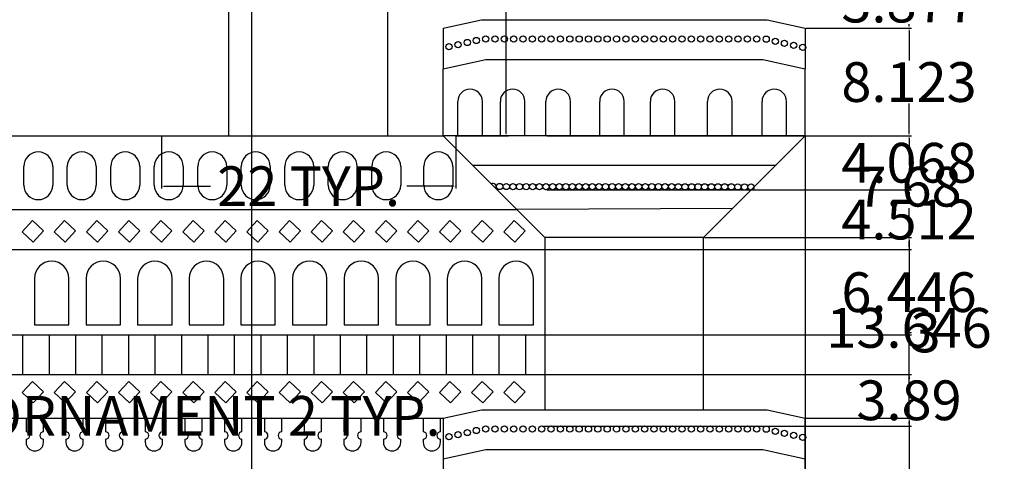
# Model space of a CAD drawing. Units: inches. Extents: x 168 to 318, y 152 to 314.
# Tile 6 of 7: x 240 to 314, y 218 to 251. Entities that reach past the tile are written whole.
import ezdxf

# ---------------------------------------------------------------- set-up
doc = ezdxf.new("R2010")
doc.units = ezdxf.units.IN
doc.header["$MEASUREMENT"] = 0
doc.layers.add('A-ANNO-DIMS', color=2, linetype='Continuous', lineweight=18)
doc.layers.add('A-ELEV', color=7, linetype='Continuous', lineweight=25)
doc.styles.get("Standard").update_dxf_attribs({"font": 'arial.ttf'})
doc.dimstyles.get("Standard").update_dxf_attribs({"dimtxt": 3, "dimasz": 0.18, "dimexe": 0.18, "dimexo": 0.0625, "dimgap": 0.09, "dimtad": 0, "dimtih": 1, "dimtoh": 1, "dimdec": 1, "dimzin": 0, "dimdsep": 46, "dimlunit": 3, "dimtxsty": 'Standard', "dimcen": 0.09, "dimadec": 0, "dimazin": 0, "dimtfac": 1, "dimtdec": 1, "dimtofl": 0, "dimtmove": 0, "dimatfit": 3, "dimfxl": 1, "dimtolj": 1, "dimtzin": 0, "dimarcsym": 0})

# ---------------------------------------------------------------- blocks, each defined once
blk = doc.blocks.new('ORN-PENDANT')
for p, q in [((0, 2.469), (0, 1.437)), ((1.31, 1.437), (1.31, 2.469)), ((0, 0.893), (0, 0.655)), ((1.31, 0.655), (1.31, 0.893))]:
    blk.add_line(p, q)
for centre, radius, start, end in [((0, 1.165), 0.272, 270, 90), ((1.31, 1.165), 0.272, 90, 270), ((0.655, 0.655), 0.655, 180, 0)]:
    blk.add_arc(centre, radius, start, end)
blk = doc.blocks.new('ARCH-BALCONY-SM')
for p, q in [((0, 0), (0, 2.603)), ((1.853, 0), (1.853, 2.603))]:
    blk.add_line(p, q)
blk.add_arc((0.926, 2.603), 0.926, 0, 180)
blk = doc.blocks.new('ARCH-ARCADE')
for p, q in [((0, 3.498), (0, 0)), ((2.6, 0), (2.6, 3.498)), ((0, 0), (2.6, 0))]:
    blk.add_line(p, q)
blk.add_arc((1.3, 3.498), 1.3, 0, 180)
blk = doc.blocks.new('OPENING-OVAL')
for p, q in [((0, 1.096), (0, 2.508)), ((2.191, 2.508), (2.191, 1.096))]:
    blk.add_line(p, q)
for centre, start, end in [((1.095, 2.508), 0, 180), ((1.095, 1.096), 180, 0)]:
    blk.add_arc(centre, 1.095, start, end)
blk = doc.blocks.new('MINARET-UPPER-STAGE')
for p, q in [((0, 24.84), (0, 22.342)), ((22.231, 24.84), (22.231, 22.343)), ((0, 18.24), (0, 22.342)), ((22.231, 18.24), (22.231, 22.342)), ((6.24, 12), (0, 18.24)), ((0, 18.24), (22.231, 18.24)), ((15.991, 12), (22.231, 18.24)), ((5.072, 0), (5.072, 12)), ((6.24, 12), (5.072, 12)), ((6.24, 12), (15.991, 12)), ((6.24, 12), (15.991, 12)), ((15.991, 12), (17.072, 12)), ((17.072, 12), (17.072, 0))]:
    blk.add_line(p, q)
for points in [[(22.231, 24.84), (19.881, 25.365), (2.344, 25.365), (0, 24.84)], [(22.231, 22.343), (19.612, 22.928), (2.613, 22.928), (0, 22.342)]]:
    blk.add_lwpolyline(points)
blk = doc.blocks.new('*D15')
at = {"layer": 'A-ANNO-DIMS', "color": 0, "lineweight": -2, "ltscale": 0.2, "transparency": 16777216}
for p, q in [((215.254, 220.875), (215.254, 221.055)), ((215.254, 221.055), (215.434, 221.055)), ((214.946, 220.875), (215.434, 220.875)), ((215.254, 218.586), (215.254, 220.695)), ((214.946, 218.406), (215.434, 218.406))]:
    blk.add_line(p, q, dxfattribs=at)
at = {"layer": 'A-ANNO-DIMS', "color": 0, "ltscale": 0.2, "transparency": 16777216}
for points in [[(215.224, 220.695), (215.284, 220.695), (215.254, 220.875)], [(215.224, 218.586), (215.284, 218.586), (215.254, 218.406)]]:
    blk.add_solid(points, dxfattribs=at)
at = {"layer": 'Defpoints', "color": 0, "ltscale": 0.2, "transparency": 16777216}
for p in [(214.883, 220.875), (215.254, 220.875), (214.883, 218.406)]:
    blk.add_point(p, dxfattribs=at)
at = {"layer": 'A-ANNO-DIMS', "color": 0, "ltscale": 0.2, "transparency": 16777216, "insert": (244.753, 221.055), "char_height": 3, "attachment_point": 5}
blk.add_mtext('\\A1;PENDANT ORNAMENT 2 TYP.', dxfattribs=at)
blk = doc.blocks.new('*D23')
at = {"layer": 'A-ANNO-DIMS', "color": 0, "lineweight": -2, "ltscale": 0.2, "transparency": 16777216}
for p, q in [((261.882, 214.562), (263.075, 214.562)), ((262.895, 214.382), (262.895, 212.619)), ((262.895, 207.574), (262.895, 209.337)), ((261.882, 207.394), (263.075, 207.394))]:
    blk.add_line(p, q, dxfattribs=at)
at = {"layer": 'A-ANNO-DIMS', "color": 0, "ltscale": 0.2, "transparency": 16777216}
for points in [[(262.865, 214.382), (262.925, 214.382), (262.895, 214.562)], [(262.865, 207.574), (262.925, 207.574), (262.895, 207.394)]]:
    blk.add_solid(points, dxfattribs=at)
at = {"layer": 'Defpoints', "color": 0, "ltscale": 0.2, "transparency": 16777216}
for p in [(261.82, 214.562), (262.895, 214.562), (261.82, 207.394)]:
    blk.add_point(p, dxfattribs=at)
at = {"layer": 'A-ANNO-DIMS', "color": 0, "ltscale": 0.2, "transparency": 16777216, "insert": (262.895, 210.978), "char_height": 3, "attachment_point": 5}
blk.add_mtext('\\A1;CUSPED ARCH PANEL 7 TYP.', dxfattribs=at)
blk = doc.blocks.new('*D25')
at = {"layer": 'A-ANNO-DIMS', "color": 0, "lineweight": -2, "ltscale": 0.2, "transparency": 16777216}
for p, q in [((273.097, 267.566), (277.02, 267.566)), ((276.84, 267.386), (276.84, 256.525)), ((276.84, 242.381), (276.84, 253.243)), ((273.097, 242.201), (277.02, 242.201))]:
    blk.add_line(p, q, dxfattribs=at)
at = {"layer": 'A-ANNO-DIMS', "color": 0, "ltscale": 0.2, "transparency": 16777216}
for points in [[(276.81, 267.386), (276.87, 267.386), (276.84, 267.566)], [(276.81, 242.381), (276.87, 242.381), (276.84, 242.201)]]:
    blk.add_solid(points, dxfattribs=at)
at = {"layer": 'Defpoints', "color": 0, "ltscale": 0.2, "transparency": 16777216}
for p in [(273.035, 267.566), (276.84, 267.566), (273.035, 242.201)]:
    blk.add_point(p, dxfattribs=at)
at = {"layer": 'A-ANNO-DIMS', "color": 0, "ltscale": 0.2, "transparency": 16777216, "insert": (276.84, 254.884), "char_height": 3, "attachment_point": 5}
blk.add_mtext('\\A1;MINARET UPPER STAGE 25 TYP.', dxfattribs=at)
blk = doc.blocks.new('*D26')
at = {"layer": 'A-ANNO-DIMS', "color": 0, "lineweight": -2, "ltscale": 0.2, "transparency": 16777216}
for p, q in [((250.804, 242.139), (250.804, 238.217)), ((273.035, 242.139), (273.035, 238.217)), ((250.984, 238.397), (254.502, 238.397)), ((272.855, 238.397), (269.337, 238.397))]:
    blk.add_line(p, q, dxfattribs=at)
at = {"layer": 'A-ANNO-DIMS', "color": 0, "ltscale": 0.2, "transparency": 16777216}
for points in [[(250.984, 238.427), (250.984, 238.367), (250.804, 238.397)], [(272.855, 238.427), (272.855, 238.367), (273.035, 238.397)]]:
    blk.add_solid(points, dxfattribs=at)
at = {"layer": 'Defpoints', "color": 0, "ltscale": 0.2, "transparency": 16777216}
for p in [(250.804, 242.201), (273.035, 242.201), (273.035, 238.397)]:
    blk.add_point(p, dxfattribs=at)
at = {"layer": 'A-ANNO-DIMS', "color": 0, "ltscale": 0.2, "transparency": 16777216, "insert": (261.92, 238.397), "char_height": 3, "attachment_point": 5}
blk.add_mtext('\\A1;22 TYP.', dxfattribs=at)
blk = doc.blocks.new('*D29')
at = {"layer": 'A-ANNO-DIMS', "color": 0, "lineweight": -2, "ltscale": 0.2, "transparency": 16777216}
for p, q in [((184.724, 242.139), (184.724, 154.215)), ((299.445, 242.139), (299.445, 154.215)), ((184.904, 154.395), (235.924, 154.395)), ((299.265, 154.395), (248.245, 154.395))]:
    blk.add_line(p, q, dxfattribs=at)
at = {"layer": 'A-ANNO-DIMS', "color": 0, "ltscale": 0.2, "transparency": 16777216}
for points in [[(184.904, 154.425), (184.904, 154.365), (184.724, 154.395)], [(299.265, 154.425), (299.265, 154.365), (299.445, 154.395)]]:
    blk.add_solid(points, dxfattribs=at)
at = {"layer": 'Defpoints', "color": 0, "ltscale": 0.2, "transparency": 16777216}
for p in [(184.724, 242.201), (299.445, 242.201), (299.445, 154.395)]:
    blk.add_point(p, dxfattribs=at)
at = {"layer": 'A-ANNO-DIMS', "color": 0, "ltscale": 0.2, "transparency": 16777216, "insert": (242.084, 154.395), "char_height": 3, "attachment_point": 5}
blk.add_mtext('\\A1;114.72', dxfattribs=at)
blk = doc.blocks.new('*D36')
at = {"layer": 'A-ANNO-DIMS', "color": 0, "lineweight": -2, "ltscale": 0.2, "transparency": 16777216}
for p, q in [((299.507, 220.875), (307.468, 220.875)), ((307.288, 220.695), (307.288, 214.997)), ((307.288, 206.055), (307.288, 211.754)), ((299.507, 205.875), (307.468, 205.875))]:
    blk.add_line(p, q, dxfattribs=at)
at = {"layer": 'A-ANNO-DIMS', "color": 0, "ltscale": 0.2, "transparency": 16777216}
for points in [[(307.258, 220.695), (307.318, 220.695), (307.288, 220.875)], [(307.258, 206.055), (307.318, 206.055), (307.288, 205.875)]]:
    blk.add_solid(points, dxfattribs=at)
at = {"layer": 'Defpoints', "color": 0, "ltscale": 0.2, "transparency": 16777216}
for p in [(299.445, 220.875), (307.288, 220.875), (299.445, 205.875)]:
    blk.add_point(p, dxfattribs=at)
at = {"layer": 'A-ANNO-DIMS', "color": 0, "ltscale": 0.2, "transparency": 16777216, "insert": (307.288, 213.375), "char_height": 3, "attachment_point": 5}
blk.add_mtext('\\A1;15', dxfattribs=at)
blk = doc.blocks.new('*D37')
at = {"layer": 'A-ANNO-DIMS', "color": 0, "lineweight": -2, "ltscale": 0.2, "transparency": 16777216}
for p, q in [((291.827, 234.521), (307.468, 234.521)), ((307.288, 234.341), (307.288, 229.321)), ((307.288, 221.055), (307.288, 226.076)), ((299.507, 220.875), (307.468, 220.875))]:
    blk.add_line(p, q, dxfattribs=at)
at = {"layer": 'A-ANNO-DIMS', "color": 0, "ltscale": 0.2, "transparency": 16777216}
for points in [[(307.258, 234.341), (307.318, 234.341), (307.288, 234.521)], [(307.258, 221.055), (307.318, 221.055), (307.288, 220.875)]]:
    blk.add_solid(points, dxfattribs=at)
at = {"layer": 'Defpoints', "color": 0, "ltscale": 0.2, "transparency": 16777216}
for p in [(291.765, 234.521), (307.288, 234.521), (299.445, 220.875)]:
    blk.add_point(p, dxfattribs=at)
at = {"layer": 'A-ANNO-DIMS', "color": 0, "ltscale": 0.2, "transparency": 16777216, "insert": (307.288, 227.698), "char_height": 3, "attachment_point": 5}
blk.add_mtext('\\A1;13.646', dxfattribs=at)
blk = doc.blocks.new('*D38')
at = {"layer": 'A-ANNO-DIMS', "color": 0, "lineweight": -2, "ltscale": 0.2, "transparency": 16777216}
for p, q in [((299.507, 242.201), (307.468, 242.201)), ((307.288, 242.021), (307.288, 239.983)), ((307.288, 234.701), (307.288, 236.74)), ((291.827, 234.521), (307.468, 234.521))]:
    blk.add_line(p, q, dxfattribs=at)
at = {"layer": 'A-ANNO-DIMS', "color": 0, "ltscale": 0.2, "transparency": 16777216}
for points in [[(307.258, 242.021), (307.318, 242.021), (307.288, 242.201)], [(307.258, 234.701), (307.318, 234.701), (307.288, 234.521)]]:
    blk.add_solid(points, dxfattribs=at)
at = {"layer": 'Defpoints', "color": 0, "ltscale": 0.2, "transparency": 16777216}
for p in [(299.445, 242.201), (307.288, 242.201), (291.765, 234.521)]:
    blk.add_point(p, dxfattribs=at)
at = {"layer": 'A-ANNO-DIMS', "color": 0, "ltscale": 0.2, "transparency": 16777216, "insert": (307.288, 238.361), "char_height": 3, "attachment_point": 5}
blk.add_mtext('\\A1;7.68', dxfattribs=at)
blk = doc.blocks.new('*D39')
at = {"layer": 'A-ANNO-DIMS', "color": 0, "lineweight": -2, "ltscale": 0.2, "transparency": 16777216}
for p, q in [((299.507, 250.324), (307.468, 250.324)), ((307.288, 250.144), (307.288, 247.886)), ((307.288, 242.381), (307.288, 244.64)), ((299.507, 242.201), (307.468, 242.201))]:
    blk.add_line(p, q, dxfattribs=at)
at = {"layer": 'A-ANNO-DIMS', "color": 0, "ltscale": 0.2, "transparency": 16777216}
for points in [[(307.258, 250.144), (307.318, 250.144), (307.288, 250.324)], [(307.258, 242.381), (307.318, 242.381), (307.288, 242.201)]]:
    blk.add_solid(points, dxfattribs=at)
at = {"layer": 'Defpoints', "color": 0, "ltscale": 0.2, "transparency": 16777216}
for p in [(299.445, 250.324), (307.288, 250.324), (299.445, 242.201)]:
    blk.add_point(p, dxfattribs=at)
at = {"layer": 'A-ANNO-DIMS', "color": 0, "ltscale": 0.2, "transparency": 16777216, "insert": (307.288, 246.263), "char_height": 3, "attachment_point": 5}
blk.add_mtext('\\A1;8.123', dxfattribs=at)
blk = doc.blocks.new('*D40')
at = {"layer": 'A-ANNO-DIMS', "color": 0, "lineweight": -2, "ltscale": 0.2, "transparency": 16777216}
for p, q in [((267.939, 254.201), (307.468, 254.201)), ((307.288, 254.021), (307.288, 253.886)), ((299.507, 250.324), (307.468, 250.324)), ((307.288, 250.504), (307.288, 250.64))]:
    blk.add_line(p, q, dxfattribs=at)
at = {"layer": 'A-ANNO-DIMS', "color": 0, "ltscale": 0.2, "transparency": 16777216}
for points in [[(307.258, 254.021), (307.318, 254.021), (307.288, 254.201)], [(307.258, 250.504), (307.318, 250.504), (307.288, 250.324)]]:
    blk.add_solid(points, dxfattribs=at)
at = {"layer": 'Defpoints', "color": 0, "ltscale": 0.2, "transparency": 16777216}
for p in [(267.877, 254.201), (307.288, 254.201), (299.445, 250.324)]:
    blk.add_point(p, dxfattribs=at)
at = {"layer": 'A-ANNO-DIMS', "color": 0, "ltscale": 0.2, "transparency": 16777216, "insert": (307.288, 252.263), "char_height": 3, "attachment_point": 5}
blk.add_mtext('\\A1;3.877', dxfattribs=at)
blk = doc.blocks.new('*D57')
at = {"layer": 'A-ANNO-DIMS', "color": 0, "lineweight": -2, "ltscale": 0.2, "transparency": 16777216}
for p, q in [((226.54, 195.647), (226.54, 312.411)), ((226.72, 312.231), (236.931, 312.231)), ((257.449, 312.231), (247.238, 312.231)), ((257.629, 195.647), (257.629, 312.411))]:
    blk.add_line(p, q, dxfattribs=at)
at = {"layer": 'A-ANNO-DIMS', "color": 0, "ltscale": 0.2, "transparency": 16777216}
for points in [[(226.72, 312.261), (226.72, 312.201), (226.54, 312.231)], [(257.449, 312.261), (257.449, 312.201), (257.629, 312.231)]]:
    blk.add_solid(points, dxfattribs=at)
at = {"layer": 'Defpoints', "color": 0, "ltscale": 0.2, "transparency": 16777216}
for p in [(257.629, 312.231), (226.54, 195.584), (257.629, 195.584)]:
    blk.add_point(p, dxfattribs=at)
at = {"layer": 'A-ANNO-DIMS', "color": 0, "ltscale": 0.2, "transparency": 16777216, "insert": (242.084, 312.231), "char_height": 3, "attachment_point": 5}
blk.add_mtext('\\A1;31.09', dxfattribs=at)
blk = doc.blocks.new('*D76')
at = {"layer": 'A-ANNO-DIMS', "color": 0, "lineweight": -2, "ltscale": 0.2, "transparency": 16777216}
for p, q in [((279.689, 220.29), (307.468, 220.29)), ((307.288, 220.11), (307.288, 215.463)), ((307.288, 207.574), (307.288, 212.22)), ((272.147, 207.394), (307.468, 207.394))]:
    blk.add_line(p, q, dxfattribs=at)
at = {"layer": 'A-ANNO-DIMS', "color": 0, "ltscale": 0.2, "transparency": 16777216}
for points in [[(307.258, 220.11), (307.318, 220.11), (307.288, 220.29)], [(307.258, 207.574), (307.318, 207.574), (307.288, 207.394)]]:
    blk.add_solid(points, dxfattribs=at)
at = {"layer": 'Defpoints', "color": 0, "ltscale": 0.2, "transparency": 16777216}
for p in [(279.627, 220.29), (307.288, 220.29), (272.084, 207.394)]:
    blk.add_point(p, dxfattribs=at)
at = {"layer": 'A-ANNO-DIMS', "color": 0, "ltscale": 0.2, "transparency": 16777216, "insert": (307.288, 213.842), "char_height": 3, "attachment_point": 5}
blk.add_mtext('\\A1;12.896', dxfattribs=at)
blk = doc.blocks.new('*D77')
at = {"layer": 'A-ANNO-DIMS', "color": 0, "lineweight": -2, "ltscale": 0.2, "transparency": 16777216}
for p, q in [((279.827, 224.175), (307.468, 224.175)), ((307.288, 223.995), (307.288, 223.855)), ((279.689, 220.29), (307.468, 220.29)), ((307.288, 220.47), (307.288, 220.61))]:
    blk.add_line(p, q, dxfattribs=at)
at = {"layer": 'A-ANNO-DIMS', "color": 0, "ltscale": 0.2, "transparency": 16777216}
for points in [[(307.258, 223.995), (307.318, 223.995), (307.288, 224.175)], [(307.258, 220.47), (307.318, 220.47), (307.288, 220.29)]]:
    blk.add_solid(points, dxfattribs=at)
at = {"layer": 'Defpoints', "color": 0, "ltscale": 0.2, "transparency": 16777216}
for p in [(279.765, 224.175), (307.288, 224.175), (279.627, 220.29)]:
    blk.add_point(p, dxfattribs=at)
at = {"layer": 'A-ANNO-DIMS', "color": 0, "ltscale": 0.2, "transparency": 16777216, "insert": (307.288, 222.232), "char_height": 3, "attachment_point": 5}
blk.add_mtext('\\A1;3.89', dxfattribs=at)
blk = doc.blocks.new('*D78')
at = {"layer": 'A-ANNO-DIMS', "color": 0, "lineweight": -2, "ltscale": 0.2, "transparency": 16777216}
for p, q in [((279.827, 227.175), (307.468, 227.175)), ((307.288, 227.175), (307.288, 227.355)), ((307.288, 227.355), (307.468, 227.355)), ((307.288, 224.355), (307.288, 226.995)), ((279.827, 224.175), (307.468, 224.175))]:
    blk.add_line(p, q, dxfattribs=at)
at = {"layer": 'A-ANNO-DIMS', "color": 0, "ltscale": 0.2, "transparency": 16777216}
for points in [[(307.258, 226.995), (307.318, 226.995), (307.288, 227.175)], [(307.258, 224.355), (307.318, 224.355), (307.288, 224.175)]]:
    blk.add_solid(points, dxfattribs=at)
at = {"layer": 'Defpoints', "color": 0, "ltscale": 0.2, "transparency": 16777216}
for p in [(279.765, 227.175), (307.288, 227.175), (279.765, 224.175)]:
    blk.add_point(p, dxfattribs=at)
at = {"layer": 'A-ANNO-DIMS', "color": 0, "ltscale": 0.2, "transparency": 16777216, "insert": (308.541, 227.355), "char_height": 3, "attachment_point": 5}
blk.add_mtext('\\A1;3', dxfattribs=at)
blk = doc.blocks.new('*D79')
at = {"layer": 'A-ANNO-DIMS', "color": 0, "lineweight": -2, "ltscale": 0.2, "transparency": 16777216}
for p, q in [((279.827, 233.621), (307.468, 233.621)), ((307.288, 233.441), (307.288, 232.02)), ((307.288, 227.355), (307.288, 228.776)), ((279.827, 227.175), (307.468, 227.175))]:
    blk.add_line(p, q, dxfattribs=at)
at = {"layer": 'A-ANNO-DIMS', "color": 0, "ltscale": 0.2, "transparency": 16777216}
for points in [[(307.258, 233.441), (307.318, 233.441), (307.288, 233.621)], [(307.258, 227.355), (307.318, 227.355), (307.288, 227.175)]]:
    blk.add_solid(points, dxfattribs=at)
at = {"layer": 'Defpoints', "color": 0, "ltscale": 0.2, "transparency": 16777216}
for p in [(279.765, 233.621), (307.288, 233.621), (279.765, 227.175)]:
    blk.add_point(p, dxfattribs=at)
at = {"layer": 'A-ANNO-DIMS', "color": 0, "ltscale": 0.2, "transparency": 16777216, "insert": (307.288, 230.398), "char_height": 3, "attachment_point": 5}
blk.add_mtext('\\A1;6.446', dxfattribs=at)
blk = doc.blocks.new('*D80')
at = {"layer": 'A-ANNO-DIMS', "color": 0, "lineweight": -2, "ltscale": 0.2, "transparency": 16777216}
for p, q in [((279.917, 238.133), (307.468, 238.133)), ((307.288, 237.953), (307.288, 237.499)), ((307.288, 233.801), (307.288, 234.255)), ((279.827, 233.621), (307.468, 233.621))]:
    blk.add_line(p, q, dxfattribs=at)
at = {"layer": 'A-ANNO-DIMS', "color": 0, "ltscale": 0.2, "transparency": 16777216}
for points in [[(307.258, 237.953), (307.318, 237.953), (307.288, 238.133)], [(307.258, 233.801), (307.318, 233.801), (307.288, 233.621)]]:
    blk.add_solid(points, dxfattribs=at)
at = {"layer": 'Defpoints', "color": 0, "ltscale": 0.2, "transparency": 16777216}
for p in [(279.854, 238.133), (307.288, 238.133), (279.765, 233.621)]:
    blk.add_point(p, dxfattribs=at)
at = {"layer": 'A-ANNO-DIMS', "color": 0, "ltscale": 0.2, "transparency": 16777216, "insert": (307.288, 235.877), "char_height": 3, "attachment_point": 5}
blk.add_mtext('\\A1;4.512', dxfattribs=at)
blk = doc.blocks.new('*D81')
at = {"layer": 'A-ANNO-DIMS', "color": 0, "lineweight": -2, "ltscale": 0.2, "transparency": 16777216}
for p, q in [((279.916, 242.201), (307.468, 242.201)), ((307.288, 242.021), (307.288, 241.789)), ((279.917, 238.133), (307.468, 238.133)), ((307.288, 238.313), (307.288, 238.545))]:
    blk.add_line(p, q, dxfattribs=at)
at = {"layer": 'A-ANNO-DIMS', "color": 0, "ltscale": 0.2, "transparency": 16777216}
for points in [[(307.258, 242.021), (307.318, 242.021), (307.288, 242.201)], [(307.258, 238.313), (307.318, 238.313), (307.288, 238.133)]]:
    blk.add_solid(points, dxfattribs=at)
at = {"layer": 'Defpoints', "color": 0, "ltscale": 0.2, "transparency": 16777216}
for p in [(279.854, 242.201), (307.288, 242.201), (279.854, 238.133)]:
    blk.add_point(p, dxfattribs=at)
at = {"layer": 'A-ANNO-DIMS', "color": 0, "ltscale": 0.2, "transparency": 16777216, "insert": (307.288, 240.167), "char_height": 3, "attachment_point": 5}
blk.add_mtext('\\A1;4.068', dxfattribs=at)

msp = doc.modelspace()

# ---------------------------------------------------------------- linework, layer by layer
at = {"layer": 'A-ELEV'}
for p, q in [((272.0845, 250.3243), (272.0845, 247.2504)), ((299.4446, 250.3243), (299.4446, 247.25)), ((272.0845, 242.2013), (272.0845, 247.25)), ((299.4446, 242.2013), (299.4446, 247.25)), ((212.0845, 242.2013), (272.0845, 242.2013)), ((299.4446, 242.2013), (272.0845, 242.2013)), ((279.7645, 234.5213), (272.0845, 242.2013)), ((291.7645, 234.5213), (299.4446, 242.2013)), ((297.2168, 239.9735), (274.3285, 239.9573)), ((206.511, 236.6279), (277.6579, 236.6279)), ((293.9532, 236.7099), (277.6579, 236.6279)), ((279.7645, 234.5213), (279.7645, 221.5213)), ((291.7645, 234.5213), (279.7645, 234.5213)), ((291.7645, 221.5213), (291.7645, 234.5213)), ((204.4044, 233.6213), (279.7645, 233.6213)), ((204.4044, 227.1751), (279.7645, 227.1751)), ((240.3013, 227.1751), (240.3013, 224.1751)), ((242.3013, 227.1751), (242.3013, 224.1751)), ((244.3013, 227.1751), (244.3013, 224.1751)), ((246.3013, 227.1751), (246.3013, 224.1751)), ((248.3013, 227.1751), (248.3013, 224.1751)), ((250.3013, 227.1751), (250.3013, 224.1751)), ((252.3013, 227.1751), (252.3013, 224.1751)), ((254.3013, 227.1751), (254.3013, 224.1751)), ((256.3013, 227.1751), (256.3013, 224.1751)), ((258.3013, 227.1751), (258.3013, 224.1751)), ((260.3013, 227.1751), (260.3013, 224.1751)), ((262.3013, 227.1751), (262.3013, 224.1751)), ((264.3013, 227.1751), (264.3013, 224.1751)), ((266.3013, 227.1751), (266.3013, 224.1751)), ((268.3013, 227.1751), (268.3013, 224.1751)), ((270.3013, 227.1751), (270.3013, 224.1751)), ((272.3013, 227.1751), (272.3013, 224.1751)), ((274.3013, 227.1751), (274.3013, 224.1751)), ((276.3013, 227.1751), (276.3013, 224.1751)), ((278.3013, 227.1751), (278.3013, 224.1751)), ((204.4044, 224.1751), (279.7645, 224.1751)), ((212.0845, 220.8755), (272.0845, 220.8755)), ((272.0845, 220.8755), (272.0845, 205.8755)), ((299.4446, 205.8755), (299.4446, 220.8755))]:
    msp.add_line(p, q, dxfattribs=at)
for points in [[(272.0845, 250.3243), (274.976, 250.9701), (296.5602, 250.9701), (299.4446, 250.3243)], [(272.0845, 247.2504), (275.3069, 247.9701), (296.2285, 247.9701), (299.4446, 247.25)], [(272.0845, 220.8755), (274.976, 221.5213), (296.5602, 221.5213), (299.4446, 220.8755)], [(272.0845, 217.8016), (275.3069, 218.5213), (296.2285, 218.5213), (299.4446, 217.8012)]]:
    msp.add_lwpolyline(points, dxfattribs=at)
for points in [[(241.8881, 235.0162), (241.0529, 235.7986), (240.2706, 234.9634), (241.1057, 234.1811)], [(244.3143, 235.0162), (243.4792, 235.7986), (242.6968, 234.9634), (243.532, 234.1811)], [(246.7406, 235.0162), (245.9054, 235.7986), (245.1231, 234.9634), (245.9582, 234.1811)], [(249.1668, 235.0162), (248.3317, 235.7986), (247.5493, 234.9634), (248.3845, 234.1811)], [(251.5931, 235.0162), (250.7579, 235.7986), (249.9756, 234.9634), (250.8108, 234.1811)], [(254.0194, 235.0162), (253.1842, 235.7986), (252.4019, 234.9634), (253.237, 234.1811)], [(256.4456, 235.0162), (255.6105, 235.7986), (254.8281, 234.9634), (255.6633, 234.1811)], [(258.8719, 235.0162), (258.0367, 235.7986), (257.2544, 234.9634), (258.0896, 234.1811)], [(261.2982, 235.0162), (260.463, 235.7986), (259.6806, 234.9634), (260.5158, 234.1811)], [(263.7244, 235.0162), (262.8892, 235.7986), (262.1069, 234.9634), (262.9421, 234.1811)], [(266.1507, 235.0162), (265.3155, 235.7986), (264.5332, 234.9634), (265.3683, 234.1811)], [(268.5769, 235.0162), (267.7418, 235.7986), (266.9594, 234.9634), (267.7946, 234.1811)], [(271.0032, 235.0162), (270.168, 235.7986), (269.3857, 234.9634), (270.2209, 234.1811)], [(273.4295, 235.0162), (272.5943, 235.7986), (271.812, 234.9634), (272.6471, 234.1811)], [(275.8557, 235.0162), (275.0206, 235.7986), (274.2382, 234.9634), (275.0734, 234.1811)], [(278.282, 235.0162), (277.4468, 235.7986), (276.6645, 234.9634), (277.4996, 234.1811)], [(241.8881, 222.8812), (241.0529, 223.6635), (240.2706, 222.8284), (241.1057, 222.046)], [(244.3143, 222.8812), (243.4792, 223.6635), (242.6968, 222.8284), (243.532, 222.046)], [(246.7406, 222.8812), (245.9054, 223.6635), (245.1231, 222.8284), (245.9582, 222.046)], [(249.1668, 222.8812), (248.3317, 223.6635), (247.5493, 222.8284), (248.3845, 222.046)], [(251.5931, 222.8812), (250.7579, 223.6635), (249.9756, 222.8284), (250.8108, 222.046)], [(254.0194, 222.8812), (253.1842, 223.6635), (252.4019, 222.8284), (253.237, 222.046)], [(256.4456, 222.8812), (255.6105, 223.6635), (254.8281, 222.8284), (255.6633, 222.046)], [(258.8719, 222.8812), (258.0367, 223.6635), (257.2544, 222.8284), (258.0896, 222.046)], [(261.2982, 222.8812), (260.463, 223.6635), (259.6806, 222.8284), (260.5158, 222.046)], [(263.7244, 222.8812), (262.8892, 223.6635), (262.1069, 222.8284), (262.9421, 222.046)], [(266.1507, 222.8812), (265.3155, 223.6635), (264.5332, 222.8284), (265.3683, 222.046)], [(268.5769, 222.8812), (267.7418, 223.6635), (266.9594, 222.8284), (267.7946, 222.046)], [(271.0032, 222.8812), (270.168, 223.6635), (269.3857, 222.8284), (270.2209, 222.046)], [(273.4295, 222.8812), (272.5943, 223.6635), (271.812, 222.8284), (272.6471, 222.046)], [(275.8557, 222.8812), (275.0206, 223.6635), (274.2382, 222.8284), (275.0734, 222.046)], [(278.282, 222.8812), (277.4468, 223.6635), (276.6645, 222.8284), (277.4996, 222.046)]]:
    msp.add_lwpolyline(points, close=True, dxfattribs=at)
for centre in [(273.2141, 249.0923), (273.9034, 249.2463), (274.5928, 249.4003), (275.2971, 249.5215), (276.0034, 249.5215), (276.7097, 249.5215), (277.4161, 249.5215), (278.1224, 249.5215), (278.8287, 249.5215), (279.535, 249.5215), (280.2414, 249.5215), (280.9477, 249.5215), (281.654, 249.5215), (282.3604, 249.5215), (283.0667, 249.5215), (283.773, 249.5215), (284.4793, 249.5215), (285.1857, 249.5215), (285.892, 249.5215), (286.5983, 249.5215), (287.3047, 249.5215), (288.011, 249.5215), (288.7173, 249.5215), (289.4236, 249.5215), (290.13, 249.5215), (290.8363, 249.5215), (291.5426, 249.5215), (292.249, 249.5215), (292.9553, 249.5215), (293.6616, 249.5215), (294.3679, 249.5215), (295.0743, 249.5215), (295.7806, 249.5215), (296.4959, 249.5001), (297.1852, 249.3457), (297.8745, 249.1914), (298.5637, 249.0371), (272.5247, 248.9384), (299.253, 248.8828), (276.354, 238.3735), (276.854, 238.3728), (277.354, 238.372), (277.854, 238.3713), (278.354, 238.3706), (278.854, 238.3699), (279.354, 238.3692), (279.854, 238.3685), (280.354, 238.3677), (280.854, 238.367), (281.354, 238.3663), (281.854, 238.3656), (282.354, 238.3649), (282.854, 238.3642), (283.354, 238.3634), (283.854, 238.3627), (284.354, 238.362), (284.854, 238.3613), (285.354, 238.3606), (285.854, 238.3599), (286.354, 238.3591), (286.854, 238.3584), (287.354, 238.3577), (287.854, 238.357), (288.354, 238.3563), (288.854, 238.3556), (289.354, 238.3548), (289.854, 238.3541), (290.354, 238.3534), (290.854, 238.3527), (291.354, 238.352), (291.854, 238.3513), (292.354, 238.3505), (292.854, 238.3498), (293.354, 238.3491), (293.854, 238.3484), (294.354, 238.3477), (294.854, 238.347), (295.354, 238.3462), (275.2971, 220.0727), (276.0034, 220.0727), (276.7097, 220.0727), (277.4161, 220.0727), (278.1224, 220.0727), (278.8287, 220.0727), (279.535, 220.0727), (280.2414, 220.0727), (280.9477, 220.0727), (281.654, 220.0727), (282.3604, 220.0727), (283.0667, 220.0727), (283.773, 220.0727), (284.4793, 220.0727), (285.1857, 220.0727), (285.892, 220.0727), (286.5983, 220.0727), (287.3047, 220.0727), (288.011, 220.0727), (288.7173, 220.0727), (289.4236, 220.0727), (290.13, 220.0727), (290.8363, 220.0727), (291.5426, 220.0727), (292.249, 220.0727), (292.9553, 220.0727), (293.6616, 220.0727), (294.3679, 220.0727), (295.0743, 220.0727), (295.7806, 220.0727), (296.4959, 220.0513), (272.5247, 219.4896), (273.2141, 219.6435), (273.9034, 219.7975), (274.5928, 219.9515), (297.1852, 219.8969), (297.8745, 219.7426), (298.5637, 219.5883), (299.253, 219.434)]:
    msp.add_circle(centre, 0.2354, dxfattribs=at)
msp.add_arc((275.854, 238.3742), 0.2354, 324.95912, 125.04088, dxfattribs=at)

# ---------------------------------------------------------------- block references
for name, p in [('MINARET-UPPER-STAGE', (250.8041, 242.2012)), ('ARCH-BALCONY-SM', (273.1935, 242.2009)), ('ARCH-BALCONY-SM', (276.4067, 242.2009)), ('ARCH-BALCONY-SM', (279.8536, 242.2009)), ('ARCH-BALCONY-SM', (283.9118, 242.2009)), ('ARCH-BALCONY-SM', (287.7406, 242.2009)), ('ARCH-BALCONY-SM', (292.0638, 242.2009)), ('ARCH-BALCONY-SM', (296.1823, 242.2009)), ('OPENING-OVAL', (240.3947, 237.381)), ('OPENING-OVAL', (243.6811, 237.381)), ('OPENING-OVAL', (246.9676, 237.381)), ('OPENING-OVAL', (250.254, 237.381)), ('OPENING-OVAL', (253.5404, 237.381)), ('OPENING-OVAL', (256.8268, 237.381)), ('OPENING-OVAL', (260.1132, 237.381)), ('OPENING-OVAL', (263.3996, 237.381)), ('OPENING-OVAL', (266.686, 237.381)), ('OPENING-OVAL', (270.6196, 237.3808)), ('ARCH-ARCADE', (241.199, 227.938)), ('ARCH-ARCADE', (245.099, 227.938)), ('ARCH-ARCADE', (248.999, 227.938)), ('ARCH-ARCADE', (252.899, 227.938)), ('ARCH-ARCADE', (256.799, 227.938)), ('ARCH-ARCADE', (260.699, 227.938)), ('ARCH-ARCADE', (264.599, 227.938)), ('ARCH-ARCADE', (268.499, 227.938)), ('ARCH-ARCADE', (272.399, 227.938)), ('ARCH-ARCADE', (276.299, 227.938)), ('ORN-PENDANT', (240.573, 218.406)), ('ORN-PENDANT', (243.573, 218.406)), ('ORN-PENDANT', (246.573, 218.406)), ('ORN-PENDANT', (249.573, 218.406)), ('ORN-PENDANT', (252.573, 218.406)), ('ORN-PENDANT', (255.573, 218.406)), ('ORN-PENDANT', (258.573, 218.406)), ('ORN-PENDANT', (261.573, 218.406)), ('ORN-PENDANT', (264.573, 218.406)), ('ORN-PENDANT', (267.573, 218.406)), ('ORN-PENDANT', (270.573, 218.406))]:
    msp.add_blockref(name, p, dxfattribs=at)

# ---------------------------------------------------------------- dimensions: what is measured, and where the dimension line sits
at = {"layer": 'A-ANNO-DIMS', "ltscale": 0.2}
for base, p1, p2, picture, middle in [((257.6286, 312.2308), (226.5403, 195.5844), (257.6286, 195.5844), '*D57', (242.0845, 312.2308)), ((299.4446, 154.3954), (184.7244, 242.2013), (299.4446, 242.2013), '*D29', (242.0845, 154.3954))]:
    dim = msp.add_linear_dim(base=base, p1=p1, p2=p2, dimstyle='Standard', override={"dimdec": 2, "dimlfac": 1, "dimrnd": 0, "dimzin": 0, "dimdsep": 46, "dimlunit": 2}, dxfattribs=at)
    dim.commit()
    dim.dimension.update_dxf_attribs({"geometry": picture, "text_midpoint": middle})
for base, p1, p2, text, picture, middle in [((276.8396, 267.5663), (273.0348, 242.2013), (273.0348, 267.5663), 'MINARET UPPER STAGE <> TYP.', '*D25', (276.8396, 254.8838)), ((215.2539, 220.8755), (214.8834, 218.4056), (214.8834, 220.8755), 'PENDANT ORNAMENT <> TYP.', '*D15', (244.7534, 221.0555)), ((262.8949, 214.5622), (261.8196, 207.3935), (261.8196, 214.5622), 'CUSPED ARCH PANEL <> TYP.', '*D23', (262.8949, 210.9778))]:
    dim = msp.add_linear_dim(base=base, p1=p1, p2=p2, angle=90, text=text, dimstyle='Standard', override={"dimdec": 0, "dimrnd": 0, "dimzin": 0, "dimlunit": 2}, dxfattribs=at)
    dim.commit()
    dim.dimension.update_dxf_attribs({"geometry": picture, "text_midpoint": middle})
for base, p1, p2, override, picture, middle in [((307.2884, 254.2013), (299.4446, 250.3243), (267.8765, 254.2013), {"dimdec": 3, "dimlfac": 1, "dimrnd": 0, "dimzin": 0, "dimdsep": 46, "dimlunit": 2}, '*D40', (307.2884, 252.2628)), ((307.2884, 250.3243), (299.4446, 242.2013), (299.4446, 250.3243), {"dimdec": 3, "dimlfac": 1, "dimrnd": 0, "dimzin": 0, "dimdsep": 46, "dimlunit": 2}, '*D39', (307.2884, 246.2628)), ((307.2884, 242.2013), (279.854, 238.133), (279.8535, 242.2013), {"dimdec": 3, "dimlfac": 1, "dimrnd": 0, "dimzin": 0, "dimdsep": 46, "dimlunit": 2}, '*D81', (307.2884, 240.1672)), ((307.2884, 242.2013), (291.7645, 234.5213), (299.4446, 242.2013), {"dimdec": 2, "dimlfac": 1, "dimrnd": 0, "dimzin": 0, "dimdsep": 46, "dimlunit": 2}, '*D38', (307.2884, 238.3613)), ((307.2884, 238.133), (279.7645, 233.6213), (279.854, 238.133), {"dimdec": 3, "dimlfac": 1, "dimrnd": 0, "dimzin": 0, "dimdsep": 46, "dimlunit": 2}, '*D80', (307.2884, 235.8772)), ((307.2884, 234.5213), (299.4446, 220.8755), (291.7645, 234.5213), {"dimdec": 3, "dimlfac": 1, "dimrnd": 0, "dimzin": 0, "dimdsep": 46, "dimlunit": 2}, '*D37', (307.2884, 227.6984)), ((307.2884, 233.6213), (279.7645, 227.1751), (279.7645, 233.6213), {"dimdec": 3, "dimlfac": 1, "dimrnd": 0, "dimzin": 0, "dimdsep": 46, "dimlunit": 2}, '*D79', (307.2884, 230.3982)), ((307.2884, 227.1751), (279.7645, 224.1751), (279.7645, 227.1751), {"dimdec": 0, "dimlfac": 1, "dimrnd": 0, "dimzin": 0, "dimdsep": 46, "dimlunit": 2}, '*D78', (308.5407, 227.3551)), ((307.2884, 224.1751), (279.6267, 220.2897), (279.7645, 224.1751), {"dimdec": 2, "dimlfac": 1, "dimrnd": 0, "dimzin": 0, "dimdsep": 46, "dimlunit": 2}, '*D77', (307.2884, 222.2324)), ((307.2884, 220.2897), (272.0845, 207.3935), (279.6267, 220.2897), {"dimdec": 3, "dimlfac": 1, "dimrnd": 0, "dimzin": 0, "dimdsep": 46, "dimlunit": 2}, '*D76', (307.2884, 213.8416)), ((307.2884, 220.8755), (299.4446, 205.8755), (299.4446, 220.8755), {"dimdec": 0, "dimlfac": 1, "dimrnd": 0, "dimzin": 0, "dimdsep": 46, "dimlunit": 2}, '*D36', (307.2884, 213.3755))]:
    dim = msp.add_linear_dim(base=base, p1=p1, p2=p2, angle=90, dimstyle='Standard', override=override, dxfattribs=at)
    dim.commit()
    dim.dimension.update_dxf_attribs({"geometry": picture, "text_midpoint": middle})
dim = msp.add_linear_dim(base=(273.0348, 238.3966), p1=(250.8042, 242.2013), p2=(273.0348, 242.2013), text='<> TYP.', dimstyle='Standard', override={"dimdec": 0, "dimrnd": 0, "dimzin": 0, "dimlunit": 2}, dxfattribs=at)
dim.commit()
dim.dimension.update_dxf_attribs({"geometry": '*D26', "text_midpoint": (261.9195, 238.3966)})

doc.saveas('drawing.dxf')
